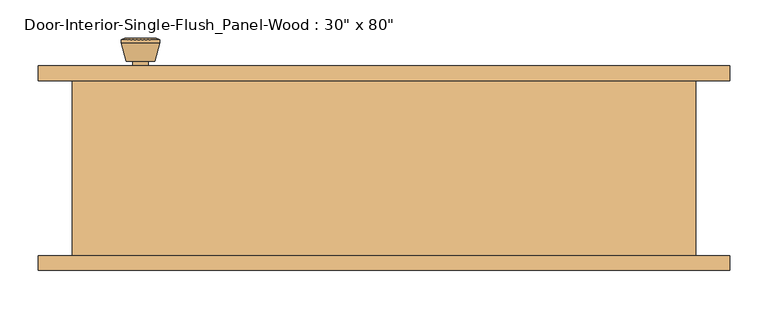
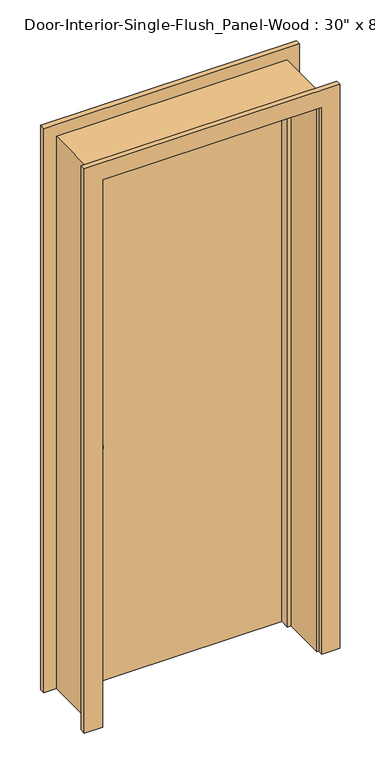
"""IFC4 building model written with IfcOpenShell, lengths in millimetres: door geometry."""

from ifc_helpers import new_model, si_unit, point, frame, frame_2d, origin, origin_with_axes, place, context, project, spatial, polyline, circle_curve, trimmed, segment, composite_curve, outline, extrude, faceted_brep, source, transform, mapped, element, save
from ifc_brep_helpers import plane_surface, cylinder_surface, revolved_surface, advanced_brep


def door_d1f25229(model_context):
    return source(origin(), model_context, "Body", "SolidModel", [
        advanced_brep(
        [(-317.5, 70.2, 914.4), (-307.5, 70.2, 914.4), (-327.5, 70.2, 914.4), (-297.0241324, 21.2, 914.4), (-317.5, 21.2, 914.4), (-337.9758676, 21.2, 914.4), (-292.5, 23.0278681, 914.4), (-342.5, 23.0278681, 914.4), (-292.5, 26.4915463, 914.4), (-342.5, 26.4915463, 914.4), (-298.863764, 51.2, 914.4), (-336.136236, 51.2, 914.4), (-307.5, 51.2, 914.4), (-327.5, 51.2, 914.4)],
        [
            (0, 1),
            (1, 2, circle_curve(frame((-317.5, 70.2, 914.4), z_axis=(0.0, 1.0, 0.0), x_axis=(-1.0, 0.0, 0.0)), 10.0)),
            (2, 0),
            (2, 1, circle_curve(frame((-317.5, 70.2, 914.4), z_axis=(0.0, 1.0, 0.0), x_axis=(-1.0, 0.0, 0.0)), 10.0)),
            (3, 4),
            (4, 5),
            (5, 3, circle_curve(frame((-317.5, 21.2, 914.4), z_axis=(0.0, -1.0, 0.0), x_axis=(-1.0, 0.0, 0.0)), 20.4758676)),
            (3, 5, circle_curve(frame((-317.5, 21.2, 914.4), z_axis=(0.0, -1.0, 0.0), x_axis=(-1.0, 0.0, 0.0)), 20.4758676)),
            (6, 3),
            (5, 7),
            (7, 6, circle_curve(frame((-317.5, 23.0278681, 914.4), z_axis=(0.0, -1.0, 0.0), x_axis=(-1.0, 0.0, 0.0)), 25.0)),
            (6, 7, circle_curve(frame((-317.5, 23.0278681, 914.4), z_axis=(0.0, -1.0, 0.0), x_axis=(-1.0, 0.0, 0.0)), 25.0)),
            (8, 6),
            (7, 9),
            (9, 8, circle_curve(frame((-317.5, 26.4915463, 914.4), z_axis=(0.0, -1.0, 0.0), x_axis=(-1.0, 0.0, 0.0)), 25.0)),
            (8, 9, circle_curve(frame((-317.5, 26.4915463, 914.4), z_axis=(0.0, -1.0, 0.0), x_axis=(-1.0, 0.0, 0.0)), 25.0)),
            (10, 8),
            (9, 11),
            (11, 10, circle_curve(frame((-317.5, 51.2, 914.4), z_axis=(0.0, -1.0, 0.0), x_axis=(-1.0, 0.0, 0.0)), 18.636236)),
            (10, 11, circle_curve(frame((-317.5, 51.2, 914.4), z_axis=(0.0, -1.0, 0.0), x_axis=(-1.0, 0.0, 0.0)), 18.636236)),
            (12, 10),
            (11, 13),
            (13, 12, circle_curve(frame((-317.5, 51.2, 914.4), z_axis=(0.0, -1.0, 0.0), x_axis=(-1.0, 0.0, 0.0)), 10.0)),
            (12, 13, circle_curve(frame((-317.5, 51.2, 914.4), z_axis=(0.0, -1.0, 0.0), x_axis=(-1.0, 0.0, 0.0)), 10.0)),
            (1, 12),
            (13, 2),
        ],
        [
            plane_surface(frame((-317.5, 70.2, 914.4), z_axis=(0.0, 1.0, 0.0), x_axis=(-1.0, 0.0, 0.0))),
            plane_surface(frame((-317.5, 21.2, 914.4), z_axis=(0.0, -1.0, 0.0), x_axis=(-1.0, 0.0, 0.0))),
            revolved_surface(polyline([(-337.9758676, 21.2, 914.4), (-342.5, 23.0278681, 914.4)]), (-317.5, 70.2, 914.4), (0.0, 1.0, 0.0)),
            cylinder_surface(frame((-317.5, 70.2, 914.4), z_axis=(0.0, 1.0, 0.0), x_axis=(-1.0, 0.0, 0.0)), 25.0),
            revolved_surface(polyline([(-342.5, 26.4915463, 914.4), (-336.136236, 51.2, 914.4)]), (-317.5, 70.2, 914.4), (0.0, 1.0, 0.0)),
            plane_surface(frame((-317.5, 51.2, 914.4), z_axis=(0.0, 1.0, 0.0), x_axis=(-1.0, 0.0, 0.0))),
            cylinder_surface(frame((-317.5, 70.2, 914.4), z_axis=(0.0, 1.0, 0.0), x_axis=(-1.0, 0.0, 0.0)), 10.0),
        ],
        [
            (0, [[1, 2, 3]]),
            (0, [[-3, 4, -1]]),
            (1, [[5, 6, 7]]),
            (1, [[-6, -5, 8]]),
            (2, [[9, -7, 10, 11]]),
            (2, [[-10, -8, -9, 12]]),
            (3, [[13, -11, 14, 15]]),
            (3, [[-14, -12, -13, 16]]),
            (4, [[17, -15, 18, 19]]),
            (4, [[-18, -16, -17, 20]]),
            (5, [[21, -19, 22, 23]]),
            (5, [[-22, -20, -21, 24]]),
            (6, [[25, -23, 26, -2]]),
            (6, [[-26, -24, -25, -4]]),
        ],
    ),
        extrude(outline(composite_curve([segment(trimmed(circle_curve(frame_2d((914.4, -317.5)), 30.0), [point((914.4, -347.5))], [point((914.4, -287.5))], False, "CARTESIAN"), True, "CONTINUOUS"), segment(trimmed(circle_curve(frame_2d((914.4, -317.5)), 30.0), [point((914.4, -287.5))], [point((914.4, -347.5))], False, "CARTESIAN"), True, "CONTINUOUS")], self_intersect=False)), frame((0.0, 70.2, 0.0), z_axis=(0.0, 1.0, 0.0), x_axis=(0.0, 0.0, 1.0)), (0.0, 0.0, 1.0), 6.0),
        advanced_brep(
        [(-317.5, 117.125, 914.4), (-327.5, 117.125, 914.4), (-307.5, 117.125, 914.4), (-297.0241324, 166.125, 914.4), (-337.9758676, 166.125, 914.4), (-317.5, 166.125, 914.4), (-292.5, 164.2971319, 914.4), (-342.5, 164.2971319, 914.4), (-292.5, 160.8334537, 914.4), (-342.5, 160.8334537, 914.4), (-298.863764, 136.125, 914.4), (-336.136236, 136.125, 914.4), (-307.5, 136.125, 914.4), (-327.5, 136.125, 914.4)],
        [
            (0, 1),
            (1, 2, circle_curve(frame((-317.5, 117.125, 914.4), z_axis=(0.0, -1.0, 0.0), x_axis=(-1.0, 0.0, 0.0)), 10.0)),
            (2, 0),
            (2, 1, circle_curve(frame((-317.5, 117.125, 914.4), z_axis=(0.0, -1.0, 0.0), x_axis=(-1.0, 0.0, 0.0)), 10.0)),
            (3, 4, circle_curve(frame((-317.5, 166.125, 914.4), z_axis=(0.0, 1.0, 0.0), x_axis=(-1.0, 0.0, 0.0)), 20.4758676)),
            (4, 5),
            (5, 3),
            (4, 3, circle_curve(frame((-317.5, 166.125, 914.4), z_axis=(0.0, 1.0, 0.0), x_axis=(-1.0, 0.0, 0.0)), 20.4758676)),
            (6, 7, circle_curve(frame((-317.5, 164.2971319, 914.4), z_axis=(0.0, 1.0, 0.0), x_axis=(-1.0, 0.0, 0.0)), 25.0)),
            (7, 4),
            (3, 6),
            (7, 6, circle_curve(frame((-317.5, 164.2971319, 914.4), z_axis=(0.0, 1.0, 0.0), x_axis=(-1.0, 0.0, 0.0)), 25.0)),
            (8, 9, circle_curve(frame((-317.5, 160.8334537, 914.4), z_axis=(0.0, 1.0, 0.0), x_axis=(-1.0, 0.0, 0.0)), 25.0)),
            (9, 7),
            (6, 8),
            (9, 8, circle_curve(frame((-317.5, 160.8334537, 914.4), z_axis=(0.0, 1.0, 0.0), x_axis=(-1.0, 0.0, 0.0)), 25.0)),
            (10, 11, circle_curve(frame((-317.5, 136.125, 914.4), z_axis=(0.0, 1.0, 0.0), x_axis=(-1.0, 0.0, 0.0)), 18.636236)),
            (11, 9),
            (8, 10),
            (11, 10, circle_curve(frame((-317.5, 136.125, 914.4), z_axis=(0.0, 1.0, 0.0), x_axis=(-1.0, 0.0, 0.0)), 18.636236)),
            (12, 13, circle_curve(frame((-317.5, 136.125, 914.4), z_axis=(0.0, 1.0, 0.0), x_axis=(-1.0, 0.0, 0.0)), 10.0)),
            (13, 11),
            (10, 12),
            (13, 12, circle_curve(frame((-317.5, 136.125, 914.4), z_axis=(0.0, 1.0, 0.0), x_axis=(-1.0, 0.0, 0.0)), 10.0)),
            (1, 13),
            (12, 2),
        ],
        [
            plane_surface(frame((-317.5, 117.125, 914.4), z_axis=(0.0, -1.0, 0.0), x_axis=(-1.0, 0.0, 0.0))),
            plane_surface(frame((-317.5, 166.125, 914.4), z_axis=(0.0, 1.0, 0.0), x_axis=(-1.0, 0.0, 0.0))),
            revolved_surface(polyline([(-337.9758676, 166.125, 914.4), (-342.5, 164.2971319, 914.4)]), (-317.5, 117.125, 914.4), (0.0, -1.0, 0.0)),
            cylinder_surface(frame((-317.5, 117.125, 914.4), z_axis=(0.0, -1.0, 0.0), x_axis=(-1.0, 0.0, 0.0)), 25.0),
            revolved_surface(polyline([(-342.5, 160.8334537, 914.4), (-336.136236, 136.125, 914.4)]), (-317.5, 117.125, 914.4), (0.0, -1.0, 0.0)),
            plane_surface(frame((-317.5, 136.125, 914.4), z_axis=(0.0, -1.0, 0.0), x_axis=(-1.0, 0.0, 0.0))),
            cylinder_surface(frame((-317.5, 117.125, 914.4), z_axis=(0.0, -1.0, 0.0), x_axis=(-1.0, 0.0, 0.0)), 10.0),
        ],
        [
            (0, [[1, 2, 3]]),
            (0, [[-3, 4, -1]]),
            (1, [[5, 6, 7]]),
            (1, [[8, -7, -6]]),
            (2, [[9, 10, -5, 11]]),
            (2, [[12, -11, -8, -10]]),
            (3, [[13, 14, -9, 15]]),
            (3, [[16, -15, -12, -14]]),
            (4, [[17, 18, -13, 19]]),
            (4, [[20, -19, -16, -18]]),
            (5, [[21, 22, -17, 23]]),
            (5, [[24, -23, -20, -22]]),
            (6, [[-2, 25, -21, 26]]),
            (6, [[-4, -26, -24, -25]]),
        ],
    ),
        extrude(outline(composite_curve([segment(trimmed(circle_curve(frame_2d((914.4, -317.5)), 30.0), [point((914.4, -347.5))], [point((914.4, -287.5))], False, "CARTESIAN"), True, "CONTINUOUS"), segment(trimmed(circle_curve(frame_2d((914.4, -317.5)), 30.0), [point((914.4, -287.5))], [point((914.4, -347.5))], False, "CARTESIAN"), True, "CONTINUOUS")], self_intersect=False)), frame((0.0, 111.125, 0.0), z_axis=(0.0, 1.0, 0.0), x_axis=(0.0, 0.0, 1.0)), (0.0, 0.0, 1.0), 6.0),
        faceted_brep([(406.4, 111.125, 0.0), (406.4, -117.475, 0.0), (381.0, -117.475, 0.0), (381.0, 41.275, 0.0), (368.3, 41.275, 0.0), (368.3, 76.2, 0.0), (381.0, 76.2, 0.0), (381.0, 111.125, 0.0), (406.4, 111.125, 2057.4), (406.4, -117.475, 2057.4), (-406.4, -117.475, 2057.4), (-406.4, -117.475, 0.0), (-381.0, -117.475, 0.0), (-381.0, -117.475, 2032.0), (381.0, -117.475, 2032.0), (381.0, 41.275, 2032.0), (-381.0, 41.275, 2032.0), (-381.0, 41.275, 0.0), (-368.3, 41.275, 0.0), (-368.3, 41.275, 2019.3), (368.3, 41.275, 2019.3), (368.3, 76.2, 2019.3), (-368.3, 76.2, 2019.3), (-368.3, 76.2, 0.0), (-381.0, 76.2, 0.0), (-381.0, 76.2, 2032.0), (381.0, 76.2, 2032.0), (381.0, 111.125, 2032.0), (-381.0, 111.125, 2032.0), (-381.0, 111.125, 0.0), (-406.4, 111.125, 0.0), (-406.4, 111.125, 2057.4)], [[[0, 1, 2, 3, 4, 5, 6, 7]], [[1, 0, 8, 9]], [[2, 1, 9, 10, 11, 12, 13, 14]], [[3, 2, 14, 15]], [[4, 3, 15, 16, 17, 18, 19, 20]], [[5, 4, 20, 21]], [[6, 5, 21, 22, 23, 24, 25, 26]], [[7, 6, 26, 27]], [[0, 7, 27, 28, 29, 30, 31, 8]], [[9, 8, 31, 10]], [[15, 14, 13, 16]], [[21, 20, 19, 22]], [[27, 26, 25, 28]], [[30, 29, 24, 23, 18, 17, 12, 11]], [[10, 31, 30, 11]], [[16, 13, 12, 17]], [[22, 19, 18, 23]], [[28, 25, 24, 29]]]),
        extrude(outline(polyline([(381.0, 76.2), (-381.0, 76.2), (-381.0, 111.125), (381.0, 111.125), (381.0, 76.2)])), origin_with_axes(), (0.0, 0.0, 1.0), 2032.0),
        extrude(outline(polyline([(0.0, 387.35), (0.0, 450.85), (2101.85, 450.85), (2101.85, -450.85), (0.0, -450.85), (0.0, -387.35), (2038.35, -387.35), (2038.35, 387.35), (0.0, 387.35)])), frame((0.0, 111.125, 0.0), z_axis=(0.0, 1.0, 0.0), x_axis=(0.0, 0.0, 1.0)), (0.0, 0.0, 1.0), 19.05),
        extrude(outline(polyline([(0.0, 387.35), (0.0, 450.85), (2101.85, 450.85), (2101.85, -450.85), (0.0, -450.85), (0.0, -387.35), (2038.35, -387.35), (2038.35, 387.35), (0.0, 387.35)])), frame((0.0, -136.525, 0.0), z_axis=(0.0, 1.0, 0.0), x_axis=(0.0, 0.0, 1.0)), (0.0, 0.0, 1.0), 19.05),
    ])


if __name__ == "__main__":
    model = new_model("IFC4")
    model_context = context("Model", 3, world=origin())
    ifc_project = project(units=[si_unit("LENGTHUNIT", "METRE", prefix="MILLI")], contexts=[model_context])
    site = spatial("IfcSite", under=ifc_project)
    building = spatial("IfcBuilding", under=site)
    placement = place(None, origin())
    door_shape = door_d1f25229(model_context)
    element("IfcDoor", 1, ObjectType="Door-Interior-Single-Flush_Panel-Wood : 30\" x 80\"", at=placement, inside=building, context=model_context, shape_type="MappedRepresentation", body=[
        mapped(door_shape, transform((0.0, 0.0, 0.0), x_axis=(1.0, 0.0, 0.0), y_axis=(0.0, 1.0, 0.0), z_axis=(0.0, 0.0, 1.0))),
    ])
    save(model, "model.ifc")

# Revit data of these elements
# Type "Door-Interior-Single-Flush_Panel-Wood : 30\" x 80\""
#   Type Mark = "12"
#   Assembly Code = "C1020300"
#   Analytic Construction = "Wooden"
#   Thickness = 0' - 1 3/8"
#   Thermal Resistance (R) = 2.5876 (h·ft²·°F)/BTU
#   Swing Angle [instance default] = 90.00°
#   Rough Width = 2' - 8"
#   Rough Height = 6' - 9"
#   Height = 6' - 8"
#   Width = 2' - 6"
#   Heat Transfer Coefficient (U) = 0.3865 BTU/(h·ft²·°F)
#   Trim Material = Cherry
#   Panel Material = Cherry
#   Frame Material = Cherry
#   Door Handle Material = Aluminum
#   Visual Light Transmittance = 0
#   Solar Heat Gain Coefficient = 0
#   Wall Closure = (empty or 0)
#   Function = (empty or 0)
# Element 1 (IfcDoor, "Door-Interior-Single-Flush_Panel-Wood : 30\" x 80\"")
#   Materials on its faces: "Cherry", "Aluminum"
# Materials
#   "Cherry": class "Wood", colour RGB 226 177 128, transparency 0, Description = "Prunus Serotina", Cost = 0
#   "Aluminum": class "Metal", colour RGB 247 247 247, transparency 0, Description = "Aluminum 6061", Cost = 0
